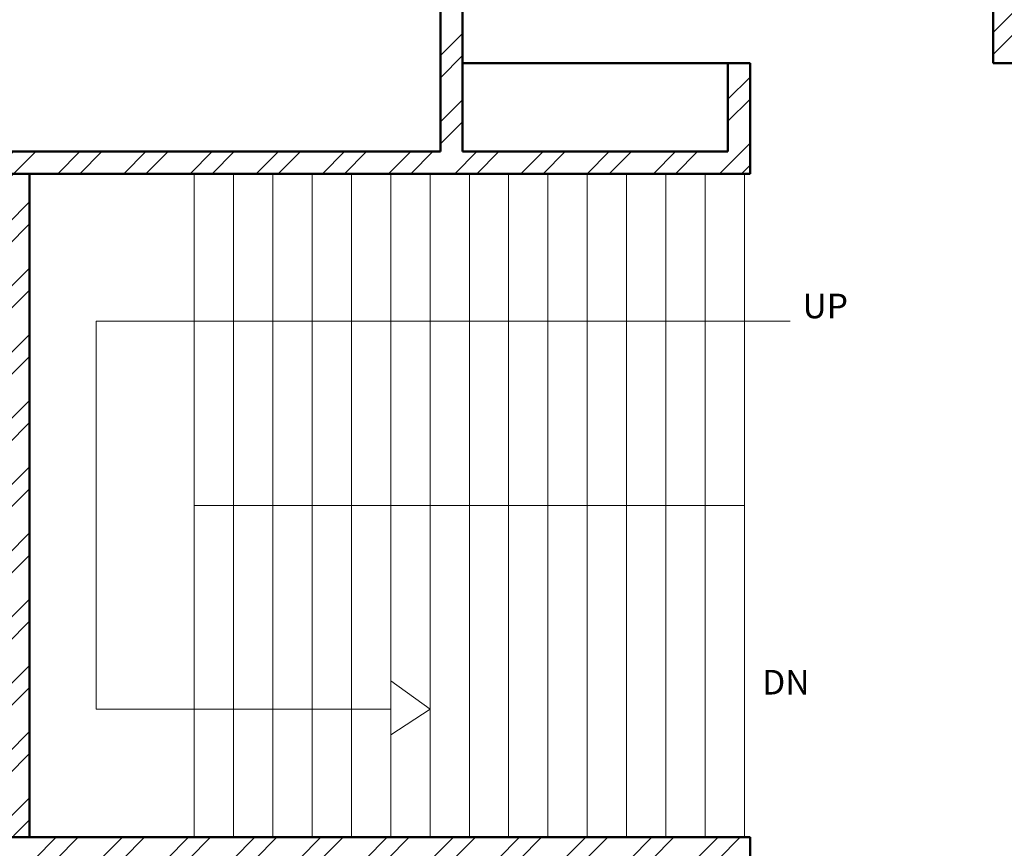
# Model space of a CAD drawing. Units: inches. Extents: x 963 to 2075, y 289 to 2657.
# Tile 29 of 98: x 1310 to 1511, y 1949 to 2117. Entities that reach past the tile are written whole.
import ezdxf

# ---------------------------------------------------------------- set-up
doc = ezdxf.new("R2010")
doc.units = ezdxf.units.IN
for name, color, linetype, lineweight in [('A-AREA-IDEN', 7, 'Continuous', 18), ('A-FLOR-STRS', 2, 'Continuous', 18), ('A-WALL', 7, 'Continuous', 50), ('A-WALL-PATT', 8, 'Continuous', 13)]:
    doc.layers.add(name, color=color, linetype=linetype, lineweight=lineweight)
doc.styles.get("Standard").update_dxf_attribs({"font": 'arial.ttf'})

msp = doc.modelspace()

# ---------------------------------------------------------------- hatches: boundary and pattern name
at = {"layer": 'A-WALL-PATT'}
h = msp.add_hatch(dxfattribs=at)
h.set_pattern_fill('ANSI32', color=256)
h.paths.add_polyline_path([(1296.92, 2558.32), (1203.92, 2558.32), (1203.92, 2493.82), (1191.53, 2493.82), (1191.53, 2489.32), (1211.06, 2489.32), (1211.06, 2492.02), (1211.06, 2493.82), (1208.42, 2493.82), (1208.42, 2553.82), (1292.42, 2553.82), (1292.42, 2538.86), (1296.92, 2538.86)])
h.paths.add_polyline_path([(1442.42, 2558.32), (1349.42, 2558.32), (1349.42, 2538.94), (1353.92, 2538.94), (1353.92, 2553.82), (1437.92, 2553.82), (1437.92, 2493.82), (1434.54, 2493.82), (1434.54, 2489.32), (1448.31, 2489.32), (1448.31, 2491.57), (1448.31, 2493.82), (1442.42, 2493.82)])
h.paths.add_polyline_path([(1415.55, 2491.57), (1415.55, 2493.82), (1340.94, 2493.82), (1340.94, 2489.32), (1371.92, 2489.32), (1371.92, 2378.32), (1367.6, 2378.32), (1367.6, 2373.82), (1371.92, 2373.82), (1371.92, 2355.19), (1376.42, 2355.19), (1376.42, 2489.32), (1415.55, 2489.32)])
h.paths.add_polyline_path([(1304.94, 2491.57), (1304.94, 2493.82), (1296.92, 2493.82), (1296.92, 2514.86), (1292.42, 2514.86), (1292.42, 2493.82), (1232.81, 2493.82), (1232.81, 2489.32), (1256.42, 2489.32), (1256.42, 2327.32), (1253.71, 2327.32), (1253.71, 2322.82), (1328.42, 2322.82), (1328.42, 2331.15), (1323.92, 2331.15), (1323.92, 2327.32), (1260.92, 2327.32), (1260.92, 2373.82), (1323.92, 2373.82), (1323.92, 2357.81), (1328.42, 2357.81), (1328.42, 2373.82), (1346.01, 2373.82), (1346.01, 2376.07), (1346.01, 2378.32), (1260.92, 2378.32), (1260.92, 2489.32), (1304.94, 2489.32)])
h.paths.add_polyline_path([(1226.65, 2327.32), (1124.42, 2327.32), (1124.42, 2347.45), (1119.92, 2347.45), (1119.92, 2322.82), (1163.42, 2322.82), (1163.42, 2305.43), (1165.67, 2305.43), (1167.92, 2305.43), (1167.92, 2322.82), (1226.65, 2322.82), (1226.65, 2325.07)])
h.paths.add_polyline_path([(1095.92, 2489.32), (1124.42, 2489.32), (1131.53, 2489.32), (1131.53, 2491.57), (1131.53, 2493.82), (1119.92, 2493.82), (1091.42, 2493.82), (1091.42, 2417.32), (1095.92, 2417.32), (1119.92, 2417.32), (1119.92, 2407.45), (1124.42, 2407.45), (1124.42, 2421.82), (1095.92, 2421.82)])
h.paths.add_polyline_path([(1512.92, 2558.32), (1508.42, 2558.32), (1508.42, 2493.82), (1503.4, 2493.82), (1503.4, 2489.32), (1508.42, 2489.32), (1508.42, 2327.32), (1376.42, 2327.32), (1376.42, 2330.27), (1371.92, 2330.27), (1371.92, 2298.74), (1376.42, 2298.74), (1376.42, 2322.82), (1508.42, 2322.82), (1508.42, 2165.32), (1504.26, 2165.32), (1504.26, 2160.82), (1508.42, 2160.82), (1508.42, 2108.32), (1512.92, 2108.32), (1512.92, 2160.82), (1516.18, 2160.82), (1516.18, 2163.07), (1516.18, 2165.32), (1512.92, 2165.32), (1512.92, 2322.82), (1644.92, 2322.82), (1644.92, 2298.74), (1649.42, 2298.74), (1649.42, 2322.82), (1649.42, 2330.94), (1647.17, 2330.94), (1644.92, 2330.94), (1644.92, 2327.32), (1512.92, 2327.32), (1512.92, 2489.32), (1516.76, 2489.32), (1516.76, 2491.57), (1516.76, 2493.82), (1512.92, 2493.82)])
h.paths.add_polyline_path([(1671.92, 2558.32), (1578.92, 2558.32), (1578.92, 2493.82), (1573.53, 2493.82), (1573.53, 2489.32), (1586.54, 2489.32), (1586.54, 2491.57), (1586.54, 2493.82), (1583.42, 2493.82), (1583.42, 2553.82), (1667.42, 2553.82), (1667.42, 2541.11), (1671.92, 2541.11)])
h.paths.add_polyline_path([(1681.26, 2493.82), (1671.92, 2493.82), (1671.92, 2517.11), (1667.42, 2517.11), (1667.42, 2493.82), (1610.22, 2493.82), (1610.22, 2489.32), (1644.92, 2489.32), (1644.92, 2357.87), (1649.42, 2357.87), (1649.42, 2373.82), (1652.2, 2373.82), (1652.2, 2375.83), (1652.2, 2378.32), (1649.42, 2378.32), (1649.42, 2489.32), (1681.26, 2489.32), (1681.26, 2491.57)])
h.paths.add_polyline_path([(1821.92, 2558.32), (1728.92, 2558.32), (1728.92, 2541), (1733.42, 2541), (1733.42, 2553.82), (1817.42, 2553.82), (1817.42, 2493.82), (1813.51, 2493.82), (1813.51, 2489.32), (1830.08, 2489.32), (1830.08, 2491.57), (1830.08, 2493.82), (1821.92, 2493.82)])
h.paths.add_polyline_path([(1794.24, 2493.82), (1717.26, 2493.82), (1717.26, 2489.32), (1760.42, 2489.32), (1760.42, 2378.32), (1674.4, 2378.32), (1674.4, 2373.82), (1692.92, 2373.82), (1692.92, 2356.95), (1697.42, 2356.95), (1697.42, 2373.82), (1760.42, 2373.82), (1760.42, 2327.32), (1697.42, 2327.32), (1697.42, 2333.34), (1692.92, 2333.34), (1692.92, 2322.82), (1768.04, 2322.82), (1768.04, 2325.07), (1768.04, 2327.32), (1764.92, 2327.32), (1764.92, 2489.32), (1794.24, 2489.32)])
h.paths.add_polyline_path([(1733.42, 2517), (1728.92, 2517), (1728.92, 2493.82), (1733.42, 2493.82)], flags=17)
h.paths.add_polyline_path([(1929.92, 2493.82), (1890.08, 2493.82), (1890.08, 2489.32), (1896.92, 2489.32), (1925.42, 2489.32), (1925.42, 2421.82), (1896.92, 2421.82), (1896.92, 2408.32), (1901.42, 2408.32), (1901.42, 2417.32), (1925.42, 2417.32), (1929.92, 2417.32)])
h.paths.add_polyline_path([(1901.42, 2348.32), (1896.92, 2348.32), (1896.92, 2327.32), (1800.42, 2327.32), (1800.42, 2322.82), (1853.42, 2322.82), (1853.42, 2309.45), (1857.92, 2309.45), (1857.92, 2322.82), (1901.42, 2322.82)])
h.paths.add_polyline_path([(1857.92, 2249.45), (1853.42, 2249.45), (1853.42, 2214.82), (1686.31, 2214.82), (1686.31, 2210.32), (1853.42, 2210.32), (1853.42, 2202.13), (1857.92, 2202.13), (1857.92, 2210.32)])
h.paths.add_polyline_path([(1857.92, 2142.13), (1853.42, 2142.13), (1853.42, 2115.42), (1841.42, 2115.42), (1841.42, 2088.53), (1841.42, 2046.95), (1845.92, 2046.95), (1845.92, 2110.92), (1905.92, 2110.92), (1905.92, 2092.52), (1910.42, 2092.52), (1910.42, 2115.42), (1857.92, 2115.42)])
h.paths.add_polyline_path([(1532.44, 1482.34), (1573.46, 1482.34), (1573.46, 1501), (1532.44, 1501)], flags=9)
h.paths.add_polyline_path([(1438.66, 1486.3), (1479.68, 1486.3), (1479.68, 1504.96), (1438.66, 1504.96)], flags=9)
h.paths.add_polyline_path([(1411.22, 1365.31), (1659.14, 1365.31), (1659.14, 1402.4), (1411.22, 1402.4)], flags=9)
h.paths.add_polyline_path([(1185.67, 2296.3), (1248.16, 2296.3), (1248.16, 2314.95), (1185.67, 2314.95)], flags=9)
h.paths.add_polyline_path([(1177.31, 2187.35), (1216.15, 2187.35), (1216.15, 2206.01), (1177.31, 2206.01)], flags=9)
h.paths.add_polyline_path([(1295.1, 1602.08), (1328.26, 1602.08), (1328.26, 1620.74), (1295.1, 1620.74)], flags=9)
h.paths.add_polyline_path([(1525.13, 2005.99), (1558.39, 2005.99), (1558.39, 2024.65), (1525.13, 2024.65)], flags=9)
h.paths.add_polyline_path([(1459.61, 1977.13), (1472.19, 1977.13), (1472.19, 1987.43), (1459.61, 1987.43)], flags=9)
h.paths.add_polyline_path([(1467.81, 2053.68), (1480.02, 2053.68), (1480.02, 2063.98), (1467.81, 2063.98)], flags=9)
h.paths.add_polyline_path([(1555.18, 2119.02), (1584.56, 2119.02), (1584.56, 2137.68), (1555.18, 2137.68)], flags=25)
h.paths.add_polyline_path([(1405.39, 2115.29), (1444.48, 2115.29), (1444.48, 2133.95), (1405.39, 2133.95)], flags=25)
h.paths.add_polyline_path([(1698.48, 2004.26), (1727.69, 2004.26), (1727.69, 2022.92), (1698.48, 2022.92)], flags=9)
h.paths.add_polyline_path([(1612.16, 1972.86), (1629.02, 1972.86), (1629.02, 1983.16), (1612.16, 1983.16)], flags=9)
h.paths.add_polyline_path([(1608.29, 2060.04), (1625.15, 2060.04), (1625.15, 2070.34), (1608.29, 2070.34)], flags=9)
h.paths.add_polyline_path([(1527.95, 1684.4), (1566.79, 1684.4), (1566.79, 1703.06), (1527.95, 1703.06)], flags=9)
h.paths.add_polyline_path([(1422.79, 1683.59), (1461.63, 1683.59), (1461.63, 1702.25), (1422.79, 1702.25)], flags=9)
h.paths.add_polyline_path([(1531.26, 1732.46), (1574.01, 1732.46), (1574.01, 1751.12), (1531.26, 1751.12)], flags=9)
h.paths.add_polyline_path([(1402.87, 1732.85), (1439.8, 1732.85), (1439.8, 1751.5), (1402.87, 1751.5)], flags=9)
h.paths.add_polyline_path([(1243.12, 1923.13), (1281.96, 1923.13), (1281.96, 1941.79), (1243.12, 1941.79)], flags=9)
h.paths.add_polyline_path([(1181.75, 1792.27), (1244.24, 1792.27), (1244.24, 1810.93), (1181.75, 1810.93)], flags=9)
h.paths.add_polyline_path([(1265.82, 1670.3), (1316.07, 1670.3), (1316.07, 1688.96), (1265.82, 1688.96)], flags=9)
h.paths.add_polyline_path([(1140.26, 1676.05), (1179.1, 1676.05), (1179.1, 1694.71), (1140.26, 1694.71)], flags=9)
h.paths.add_polyline_path([(1107.49, 1490.89), (1143.37, 1490.89), (1143.37, 1509.55), (1107.49, 1509.55)], flags=9)
h.paths.add_polyline_path([(1217.58, 1483.9), (1246.74, 1483.9), (1246.74, 1502.56), (1217.58, 1502.56)], flags=9)
h.paths.add_polyline_path([(1389.21, 1486.92), (1418.37, 1486.92), (1418.37, 1505.58), (1389.21, 1505.58)], flags=9)
h.paths.add_polyline_path([(1672.21, 1602.08), (1705.37, 1602.08), (1705.37, 1620.74), (1672.21, 1620.74)], flags=9)
h.paths.add_polyline_path([(1752.08, 1522.64), (1781.24, 1522.64), (1781.24, 1541.3), (1752.08, 1541.3)], flags=9)
h.paths.add_polyline_path([(1848.27, 1491.26), (1884.16, 1491.26), (1884.16, 1509.92), (1848.27, 1509.92)], flags=9)
h.paths.add_polyline_path([(1822.47, 1685.62), (1861.31, 1685.62), (1861.31, 1704.28), (1822.47, 1704.28)], flags=9)
h.paths.add_polyline_path([(1713.19, 1672.23), (1763.44, 1672.23), (1763.44, 1690.89), (1713.19, 1690.89)], flags=9)
h.paths.add_polyline_path([(1736.62, 1790.58), (1799.11, 1790.58), (1799.11, 1809.24), (1736.62, 1809.24)], flags=9)
h.paths.add_polyline_path([(1691.49, 1916.36), (1730.33, 1916.36), (1730.33, 1935.01), (1691.49, 1935.01)], flags=9)
h.paths.add_polyline_path([(1764.87, 1973.92), (1794.31, 1973.92), (1794.31, 1992.58), (1764.87, 1992.58)], flags=9)
h.paths.add_polyline_path([(1767.85, 2034.02), (1797.29, 2034.02), (1797.29, 2052.67), (1767.85, 2052.67)], flags=9)
h.paths.add_polyline_path([(1851.59, 2060.33), (1880.75, 2060.33), (1880.75, 2078.99), (1851.59, 2078.99)], flags=25)
h.paths.add_polyline_path([(1688.49, 2086.87), (1727.33, 2086.87), (1727.33, 2105.53), (1688.49, 2105.53)], flags=9)
h.paths.add_polyline_path([(1537.74, 2293.58), (1580.49, 2293.58), (1580.49, 2312.24), (1537.74, 2312.24)], flags=25)
h.paths.add_polyline_path([(1425.59, 2296.11), (1468.34, 2296.11), (1468.34, 2314.77), (1425.59, 2314.77)], flags=25)
h.paths.add_polyline_path([(1278.52, 2004.18), (1307.72, 2004.18), (1307.72, 2022.84), (1278.52, 2022.84)], flags=9)
h.paths.add_polyline_path([(1193.28, 1973.63), (1222.72, 1973.63), (1222.72, 1992.29), (1193.28, 1992.29)], flags=9)
h.paths.add_polyline_path([(1192.41, 2040.58), (1221.84, 2040.58), (1221.84, 2059.23), (1192.41, 2059.23)], flags=9)
h.paths.add_polyline_path([(1130.6, 1951.39), (1159.76, 1951.39), (1159.76, 1970.05), (1130.6, 1970.05)], flags=9)
h.paths.add_polyline_path([(1132.83, 2052.49), (1161.98, 2052.49), (1161.98, 2071.15), (1132.83, 2071.15)], flags=9)
h.paths.add_polyline_path([(1265.13, 2334.62), (1315.38, 2334.62), (1315.38, 2353.28), (1265.13, 2353.28)], flags=25)
h.paths.add_polyline_path([(1136.74, 2330.79), (1175.58, 2330.79), (1175.58, 2349.44), (1136.74, 2349.44)], flags=9)
h.paths.add_polyline_path([(1287.42, 2417.2), (1320.58, 2417.2), (1320.58, 2435.86), (1287.42, 2435.86)], flags=25)
h.paths.add_polyline_path([(1430.99, 2329.16), (1469.83, 2329.16), (1469.83, 2347.82), (1430.99, 2347.82)], flags=25)
h.paths.add_polyline_path([(1525.42, 2329.21), (1564.26, 2329.21), (1564.26, 2347.87), (1525.42, 2347.87)], flags=25)
h.paths.add_polyline_path([(1684.52, 2382.8), (1717.68, 2382.8), (1717.68, 2401.46), (1684.52, 2401.46)], flags=25)
h.paths.add_polyline_path([(1704.81, 2340.29), (1755.05, 2340.29), (1755.05, 2358.95), (1704.81, 2358.95)], flags=25)
h.paths.add_polyline_path([(1694.11, 2287.76), (1756.6, 2287.76), (1756.6, 2306.41), (1694.11, 2306.41)], flags=9)
h.paths.add_polyline_path([(1815.78, 2329.86), (1854.62, 2329.86), (1854.62, 2348.52), (1815.78, 2348.52)], flags=9)
h.paths.add_polyline_path([(1842.87, 2514.26), (1878.76, 2514.26), (1878.76, 2532.91), (1842.87, 2532.91)], flags=9)
h.paths.add_polyline_path([(1769.51, 2531.45), (1798.67, 2531.45), (1798.67, 2550.1), (1769.51, 2550.1)], flags=25)
h.paths.add_polyline_path([(1594.77, 2518.47), (1623.93, 2518.47), (1623.93, 2537.13), (1594.77, 2537.13)], flags=25)
h.paths.add_polyline_path([(1520.72, 2516.18), (1556.61, 2516.18), (1556.61, 2534.84), (1520.72, 2534.84)], flags=25)
h.paths.add_polyline_path([(1464.46, 2516.69), (1500.34, 2516.69), (1500.34, 2535.35), (1464.46, 2535.35)], flags=25)
h.paths.add_polyline_path([(1365.7, 2528.97), (1394.85, 2528.97), (1394.85, 2547.63), (1365.7, 2547.63)], flags=25)
h.paths.add_polyline_path([(1222.84, 2516.23), (1252, 2516.23), (1252, 2534.89), (1222.84, 2534.89)], flags=25)
h.paths.add_polyline_path([(1104.55, 2509.6), (1140.43, 2509.6), (1140.43, 2528.26), (1104.55, 2528.26)], flags=9)
h = msp.add_hatch(dxfattribs=at)
h.set_pattern_fill('ANSI32', color=256)
h.paths.add_polyline_path([(1335.97, 2212.57), (1335.97, 2214.82), (1167.92, 2214.82), (1167.92, 2245.43), (1163.42, 2245.43), (1163.42, 2210.32), (1163.42, 2194.81), (1167.92, 2194.81), (1167.92, 2210.32), (1335.97, 2210.32)])
h.paths.add_polyline_path([(1532.44, 1482.34), (1573.46, 1482.34), (1573.46, 1501), (1532.44, 1501)], flags=9)
h.paths.add_polyline_path([(1438.66, 1486.3), (1479.68, 1486.3), (1479.68, 1504.96), (1438.66, 1504.96)], flags=9)
h.paths.add_polyline_path([(1411.22, 1365.31), (1659.14, 1365.31), (1659.14, 1402.4), (1411.22, 1402.4)], flags=9)
h.paths.add_polyline_path([(1185.67, 2296.3), (1248.16, 2296.3), (1248.16, 2314.95), (1185.67, 2314.95)], flags=9)
h.paths.add_polyline_path([(1177.31, 2187.35), (1216.15, 2187.35), (1216.15, 2206.01), (1177.31, 2206.01)], flags=9)
h.paths.add_polyline_path([(1295.1, 1602.08), (1328.26, 1602.08), (1328.26, 1620.74), (1295.1, 1620.74)], flags=9)
h.paths.add_polyline_path([(1525.13, 2005.99), (1558.39, 2005.99), (1558.39, 2024.65), (1525.13, 2024.65)], flags=9)
h.paths.add_polyline_path([(1459.61, 1977.13), (1472.19, 1977.13), (1472.19, 1987.43), (1459.61, 1987.43)], flags=9)
h.paths.add_polyline_path([(1467.81, 2053.68), (1480.02, 2053.68), (1480.02, 2063.98), (1467.81, 2063.98)], flags=9)
h.paths.add_polyline_path([(1555.18, 2119.02), (1584.56, 2119.02), (1584.56, 2137.68), (1555.18, 2137.68)], flags=9)
h.paths.add_polyline_path([(1405.39, 2115.29), (1444.48, 2115.29), (1444.48, 2133.95), (1405.39, 2133.95)], flags=9)
h.paths.add_polyline_path([(1698.48, 2004.26), (1727.69, 2004.26), (1727.69, 2022.92), (1698.48, 2022.92)], flags=9)
h.paths.add_polyline_path([(1612.16, 1972.86), (1629.02, 1972.86), (1629.02, 1983.16), (1612.16, 1983.16)], flags=9)
h.paths.add_polyline_path([(1608.29, 2060.04), (1625.15, 2060.04), (1625.15, 2070.34), (1608.29, 2070.34)], flags=9)
h.paths.add_polyline_path([(1527.95, 1684.4), (1566.79, 1684.4), (1566.79, 1703.06), (1527.95, 1703.06)], flags=9)
h.paths.add_polyline_path([(1422.79, 1683.59), (1461.63, 1683.59), (1461.63, 1702.25), (1422.79, 1702.25)], flags=9)
h.paths.add_polyline_path([(1531.26, 1732.46), (1574.01, 1732.46), (1574.01, 1751.12), (1531.26, 1751.12)], flags=9)
h.paths.add_polyline_path([(1402.87, 1732.85), (1439.8, 1732.85), (1439.8, 1751.5), (1402.87, 1751.5)], flags=9)
h.paths.add_polyline_path([(1243.12, 1923.13), (1281.96, 1923.13), (1281.96, 1941.79), (1243.12, 1941.79)], flags=9)
h.paths.add_polyline_path([(1181.75, 1792.27), (1244.24, 1792.27), (1244.24, 1810.93), (1181.75, 1810.93)], flags=9)
h.paths.add_polyline_path([(1265.82, 1670.3), (1316.07, 1670.3), (1316.07, 1688.96), (1265.82, 1688.96)], flags=9)
h.paths.add_polyline_path([(1140.26, 1676.05), (1179.1, 1676.05), (1179.1, 1694.71), (1140.26, 1694.71)], flags=9)
h.paths.add_polyline_path([(1107.49, 1490.89), (1143.37, 1490.89), (1143.37, 1509.55), (1107.49, 1509.55)], flags=9)
h.paths.add_polyline_path([(1217.58, 1483.9), (1246.74, 1483.9), (1246.74, 1502.56), (1217.58, 1502.56)], flags=9)
h.paths.add_polyline_path([(1389.21, 1486.92), (1418.37, 1486.92), (1418.37, 1505.58), (1389.21, 1505.58)], flags=9)
h.paths.add_polyline_path([(1672.21, 1602.08), (1705.37, 1602.08), (1705.37, 1620.74), (1672.21, 1620.74)], flags=9)
h.paths.add_polyline_path([(1752.08, 1522.64), (1781.24, 1522.64), (1781.24, 1541.3), (1752.08, 1541.3)], flags=9)
h.paths.add_polyline_path([(1848.27, 1491.26), (1884.16, 1491.26), (1884.16, 1509.92), (1848.27, 1509.92)], flags=9)
h.paths.add_polyline_path([(1822.47, 1685.62), (1861.31, 1685.62), (1861.31, 1704.28), (1822.47, 1704.28)], flags=9)
h.paths.add_polyline_path([(1713.19, 1672.23), (1763.44, 1672.23), (1763.44, 1690.89), (1713.19, 1690.89)], flags=9)
h.paths.add_polyline_path([(1736.62, 1790.58), (1799.11, 1790.58), (1799.11, 1809.24), (1736.62, 1809.24)], flags=9)
h.paths.add_polyline_path([(1691.49, 1916.36), (1730.33, 1916.36), (1730.33, 1935.01), (1691.49, 1935.01)], flags=9)
h.paths.add_polyline_path([(1764.87, 1973.92), (1794.31, 1973.92), (1794.31, 1992.58), (1764.87, 1992.58)], flags=9)
h.paths.add_polyline_path([(1767.85, 2034.02), (1797.29, 2034.02), (1797.29, 2052.67), (1767.85, 2052.67)], flags=9)
h.paths.add_polyline_path([(1851.59, 2060.33), (1880.75, 2060.33), (1880.75, 2078.99), (1851.59, 2078.99)], flags=9)
h.paths.add_polyline_path([(1688.49, 2086.87), (1727.33, 2086.87), (1727.33, 2105.53), (1688.49, 2105.53)], flags=9)
h.paths.add_polyline_path([(1537.74, 2293.58), (1580.49, 2293.58), (1580.49, 2312.24), (1537.74, 2312.24)], flags=9)
h.paths.add_polyline_path([(1425.59, 2296.11), (1468.34, 2296.11), (1468.34, 2314.77), (1425.59, 2314.77)], flags=9)
h.paths.add_polyline_path([(1278.52, 2004.18), (1307.72, 2004.18), (1307.72, 2022.84), (1278.52, 2022.84)], flags=9)
h.paths.add_polyline_path([(1193.28, 1973.63), (1222.72, 1973.63), (1222.72, 1992.29), (1193.28, 1992.29)], flags=9)
h.paths.add_polyline_path([(1192.41, 2040.58), (1221.84, 2040.58), (1221.84, 2059.23), (1192.41, 2059.23)], flags=9)
h.paths.add_polyline_path([(1130.6, 1951.39), (1159.76, 1951.39), (1159.76, 1970.05), (1130.6, 1970.05)], flags=9)
h.paths.add_polyline_path([(1132.83, 2052.49), (1161.98, 2052.49), (1161.98, 2071.15), (1132.83, 2071.15)], flags=9)
h.paths.add_polyline_path([(1265.13, 2334.62), (1315.38, 2334.62), (1315.38, 2353.28), (1265.13, 2353.28)], flags=9)
h.paths.add_polyline_path([(1136.74, 2330.79), (1175.58, 2330.79), (1175.58, 2349.44), (1136.74, 2349.44)], flags=9)
h.paths.add_polyline_path([(1287.42, 2417.2), (1320.58, 2417.2), (1320.58, 2435.86), (1287.42, 2435.86)], flags=9)
h.paths.add_polyline_path([(1430.99, 2329.16), (1469.83, 2329.16), (1469.83, 2347.82), (1430.99, 2347.82)], flags=9)
h.paths.add_polyline_path([(1525.42, 2329.21), (1564.26, 2329.21), (1564.26, 2347.87), (1525.42, 2347.87)], flags=9)
h.paths.add_polyline_path([(1684.52, 2382.8), (1717.68, 2382.8), (1717.68, 2401.46), (1684.52, 2401.46)], flags=9)
h.paths.add_polyline_path([(1704.81, 2340.29), (1755.05, 2340.29), (1755.05, 2358.95), (1704.81, 2358.95)], flags=9)
h.paths.add_polyline_path([(1694.11, 2287.76), (1756.6, 2287.76), (1756.6, 2306.41), (1694.11, 2306.41)], flags=9)
h.paths.add_polyline_path([(1815.78, 2329.86), (1854.62, 2329.86), (1854.62, 2348.52), (1815.78, 2348.52)], flags=9)
h.paths.add_polyline_path([(1842.87, 2514.26), (1878.76, 2514.26), (1878.76, 2532.91), (1842.87, 2532.91)], flags=9)
h.paths.add_polyline_path([(1769.51, 2531.45), (1798.67, 2531.45), (1798.67, 2550.1), (1769.51, 2550.1)], flags=9)
h.paths.add_polyline_path([(1594.77, 2518.47), (1623.93, 2518.47), (1623.93, 2537.13), (1594.77, 2537.13)], flags=9)
h.paths.add_polyline_path([(1520.72, 2516.18), (1556.61, 2516.18), (1556.61, 2534.84), (1520.72, 2534.84)], flags=9)
h.paths.add_polyline_path([(1464.46, 2516.69), (1500.34, 2516.69), (1500.34, 2535.35), (1464.46, 2535.35)], flags=9)
h.paths.add_polyline_path([(1365.7, 2528.97), (1394.85, 2528.97), (1394.85, 2547.63), (1365.7, 2547.63)], flags=9)
h.paths.add_polyline_path([(1222.84, 2516.23), (1252, 2516.23), (1252, 2534.89), (1222.84, 2534.89)], flags=9)
h.paths.add_polyline_path([(1104.55, 2509.6), (1140.43, 2509.6), (1140.43, 2528.26), (1104.55, 2528.26)], flags=9)
h = msp.add_hatch(dxfattribs=at)
h.set_pattern_fill('ANSI32', color=256)
h.paths.add_polyline_path([(1473.61, 2163.07), (1473.61, 2165.32), (1376.42, 2165.32), (1376.42, 2227.98), (1371.92, 2227.98), (1371.92, 2214.82), (1368.41, 2214.82), (1368.41, 2210.32), (1371.92, 2210.32), (1371.92, 2160.82), (1395.92, 2160.82), (1395.92, 2090.32), (1217.34, 2090.32), (1217.34, 2085.82), (1395.92, 2085.82), (1458.92, 2085.82), (1458.92, 2108.32), (1454.42, 2108.32), (1454.42, 2090.32), (1400.42, 2090.32), (1400.42, 2160.82), (1473.61, 2160.82)])
h.paths.add_polyline_path([(1649.42, 2210.32), (1653.23, 2210.32), (1653.23, 2214.82), (1649.42, 2214.82), (1649.42, 2227.98), (1644.92, 2227.98), (1644.92, 2165.32), (1550.1, 2165.32), (1550.1, 2160.82), (1620.92, 2160.82), (1620.92, 2112.82), (1555.45, 2112.82), (1555.45, 2108.32), (1584.33, 2108.32), (1584.33, 2084.92), (1588.83, 2084.92), (1588.83, 2108.32), (1625.42, 2108.32), (1667.95, 2108.32), (1667.95, 2022.67), (1588.83, 2022.67), (1588.83, 2047.41), (1584.33, 2047.41), (1584.33, 1996), (1588.83, 1996), (1588.83, 2018.32), (1667.95, 2018.17), (1667.95, 1928.32), (1625.42, 1928.32), (1625.42, 1923.82), (1672.45, 1923.82), (1672.45, 1928.32), (1672.45, 1946.66), (1785.45, 1946.66), (1785.45, 1951.16), (1743.03, 1951.16), (1743.03, 2017.92), (1841.42, 2017.92), (1841.42, 2014.77), (1845.92, 2014.77), (1845.92, 2017.92), (1905.92, 2017.92), (1905.92, 1987.51), (1910.42, 1987.51), (1910.42, 2022.42), (1910.42, 2068.52), (1905.92, 2068.52), (1905.92, 2022.42), (1845.92, 2022.42), (1845.92, 2025.85), (1843.67, 2025.85), (1841.42, 2025.85), (1841.42, 2022.42), (1743.03, 2022.42), (1743.03, 2084.03), (1768.45, 2084.03), (1785.45, 2084.03), (1785.45, 2088.53), (1672.45, 2088.53), (1672.45, 2112.82), (1667.95, 2112.82), (1625.42, 2112.82), (1625.42, 2160.82), (1649.42, 2160.82)])
h.paths.add_polyline_path([(1672.45, 2084.03), (1738.53, 2084.03), (1738.53, 1951.16), (1672.45, 1951.16)], flags=16)
h.paths.add_polyline_path([(1672.45, 2084.03), (1738.53, 2084.03), (1705.49, 2017.6)], flags=0)
h.paths.add_polyline_path([(1262.77, 2085.82), (1258.27, 2085.82), (1258.27, 2023.28), (1184.42, 2023.28), (1184.42, 2018.78), (1258.27, 2018.78), (1258.27, 1950.82), (1262.77, 1950.82)])
h.paths.add_polyline_path([(1312.27, 2085.82), (1307.77, 2085.82), (1307.77, 1950.82), (1312.27, 1950.82)])
h.paths.add_polyline_path([(1458.92, 1950.82), (1395.92, 1950.82), (1216.57, 1950.82), (1216.57, 1946.32), (1346.42, 1946.32), (1395.92, 1946.32), (1395.92, 1875.82), (1371.92, 1875.82), (1371.92, 1826.32), (1368.93, 1826.32), (1368.93, 1821.82), (1371.92, 1821.82), (1371.92, 1813.62), (1376.42, 1813.62), (1376.42, 1871.32), (1474.5, 1871.32), (1474.5, 1873.57), (1474.5, 1875.82), (1400.42, 1875.82), (1400.42, 1946.32), (1454.42, 1946.32), (1454.42, 1928.32), (1458.92, 1928.32)])
h.paths.add_polyline_path([(1184.42, 2120.78), (1167.92, 2120.78), (1167.92, 2134.81), (1165.67, 2134.81), (1163.42, 2134.81), (1163.42, 2120.78), (1119.92, 2120.78), (1119.92, 2098.1), (1124.42, 2098.1), (1124.42, 2116.28), (1167.92, 2116.28), (1179.92, 2116.28), (1179.92, 2045.92), (1184.42, 2045.92), (1184.42, 2090.32), (1184.42, 2116.28)])
h.paths.add_polyline_path([(1124.42, 2018.78), (1179.92, 2018.78), (1179.92, 2016.29), (1184.42, 2016.29), (1184.42, 2023.28), (1184.42, 2026.59), (1182.17, 2026.59), (1179.92, 2026.59), (1179.92, 2023.28), (1124.42, 2023.28), (1124.42, 2074.1), (1119.92, 2074.1), (1119.92, 2018.78), (1119.92, 1979.63), (1124.42, 1979.63)])
h.paths.add_polyline_path([(1184.42, 1925.78), (1184.42, 1946.32), (1184.42, 1996.07), (1182.17, 1996.07), (1179.92, 1996.07), (1179.92, 1925.78), (1124.42, 1925.78), (1124.42, 1955.63), (1119.92, 1955.5), (1119.92, 1921.28), (1158.92, 1921.28), (1158.92, 1909.98), (1163.42, 1909.98), (1163.42, 1921.28), (1184.42, 1921.28)])
h.paths.add_polyline_path([(1341.45, 1826.32), (1163.42, 1826.32), (1163.42, 1849.98), (1158.92, 1849.98), (1158.92, 1821.82), (1158.92, 1804.03), (1163.42, 1804.03), (1163.42, 1821.82), (1341.45, 1821.82)])
h.paths.add_polyline_path([(1222.98, 1713.82), (1163.42, 1713.82), (1163.42, 1744.03), (1161.17, 1744.03), (1158.92, 1744.03), (1158.92, 1713.82), (1119.92, 1713.82), (1119.92, 1694.65), (1124.42, 1694.65), (1124.42, 1709.32), (1158.92, 1709.32), (1222.98, 1709.32)])
h.paths.add_polyline_path([(1328.42, 1713.82), (1252.04, 1713.82), (1252.04, 1711.57), (1252.04, 1709.32), (1256.42, 1709.32), (1256.42, 1547.32), (1232.94, 1547.32), (1232.94, 1545.07), (1232.94, 1542.82), (1292.42, 1542.82), (1292.42, 1527.63), (1296.92, 1527.63), (1296.92, 1542.82), (1299.46, 1542.82), (1299.46, 1547.32), (1260.92, 1547.32), (1260.92, 1658.32), (1343.66, 1658.32), (1343.66, 1660.57), (1343.66, 1662.82), (1328.42, 1662.82), (1328.42, 1676.59), (1327.4, 1676.59), (1323.92, 1676.59), (1323.92, 1662.82), (1260.92, 1662.82), (1260.92, 1709.32), (1323.92, 1709.32), (1323.92, 1699.85), (1328.42, 1699.85)])
h.paths.add_polyline_path([(1649.42, 1875.82), (1625.42, 1875.82), (1625.42, 1928.32), (1620.92, 1928.32), (1588.83, 1928.32), (1588.83, 1950.59), (1584.33, 1950.59), (1584.33, 1928.32), (1555.45, 1928.32), (1555.45, 1923.82), (1620.92, 1923.82), (1620.92, 1875.82), (1548.95, 1875.82), (1548.95, 1873.57), (1548.95, 1871.32), (1644.92, 1871.32), (1644.92, 1813.62), (1649.42, 1813.62), (1649.42, 1821.82), (1652.04, 1821.82), (1652.04, 1824.07), (1652.04, 1826.32), (1649.42, 1826.32)])
h.paths.add_polyline_path([(1512.92, 1871.32), (1516.48, 1871.32), (1516.48, 1875.82), (1512.92, 1875.82), (1512.92, 1923.82), (1512.92, 1928.32), (1512.92, 1930.83), (1508.42, 1930.83), (1508.42, 1875.82), (1504.41, 1875.82), (1504.41, 1871.32), (1508.42, 1871.32), (1508.42, 1713.82), (1376.42, 1713.82), (1376.42, 1743.32), (1371.92, 1743.32), (1371.92, 1709.32), (1371.92, 1706.01), (1376.42, 1706.01), (1376.42, 1709.32), (1508.42, 1709.32), (1508.42, 1547.32), (1501.87, 1547.32), (1501.87, 1542.82), (1508.42, 1542.82), (1508.42, 1482.82), (1508.42, 1436.32), (1512.92, 1436.32), (1512.92, 1542.82), (1519.32, 1542.82), (1519.32, 1545.07), (1519.32, 1547.32), (1512.92, 1547.32), (1512.92, 1709.32), (1644.92, 1709.32), (1644.92, 1707.55), (1649.42, 1707.55), (1649.42, 1709.32), (1649.42, 1743.32), (1644.92, 1743.32), (1644.92, 1713.82), (1512.92, 1713.82)])
h.paths.add_polyline_path([(1129.88, 1545.07), (1129.88, 1547.32), (1124.42, 1547.32), (1095.92, 1547.32), (1095.92, 1614.82), (1124.42, 1614.82), (1124.42, 1619.32), (1095.92, 1619.32), (1091.42, 1619.32), (1091.42, 1542.82), (1095.92, 1542.82), (1119.92, 1542.82), (1129.88, 1542.82)])
h.paths.add_polyline_path([(1208.42, 1542.82), (1211.74, 1542.82), (1211.74, 1547.32), (1198.85, 1547.32), (1198.85, 1542.82), (1203.92, 1542.82), (1203.92, 1478.32), (1208.42, 1478.32), (1296.92, 1478.32), (1296.92, 1503.63), (1292.42, 1503.63), (1292.42, 1482.82), (1208.42, 1482.82)])
h.paths.add_polyline_path([(1430.42, 1542.82), (1435.7, 1542.82), (1435.7, 1545.07), (1435.7, 1547.32), (1422.66, 1547.32), (1422.66, 1545.07), (1422.66, 1542.82), (1425.92, 1542.82), (1425.92, 1482.86), (1341.92, 1482.86), (1341.92, 1502.73), (1337.42, 1502.73), (1337.42, 1478.36), (1425.92, 1478.36), (1425.92, 1440.82), (1425.92, 1436.32), (1430.42, 1436.32)])
h.paths.add_polyline_path([(1698.48, 2004.26), (1727.69, 2004.26), (1727.69, 2022.92), (1698.48, 2022.92)], flags=8)

# ---------------------------------------------------------------- linework, layer by layer
at = {"layer": 'A-FLOR-STRS'}
for p, q in [((1345.79, 2085.82), (1345.79, 1950.82)), ((1353.79, 2085.82), (1353.79, 1950.82)), ((1361.79, 2085.82), (1361.79, 1950.82)), ((1369.79, 2085.82), (1369.79, 1950.82)), ((1377.79, 2085.82), (1377.79, 1950.82)), ((1385.79, 2085.82), (1385.79, 1950.82)), ((1393.79, 2085.82), (1393.79, 1950.82)), ((1401.79, 2085.82), (1401.79, 1950.82)), ((1409.79, 2085.82), (1409.79, 1950.82)), ((1417.79, 2085.82), (1417.79, 1950.82)), ((1425.79, 2085.82), (1425.79, 1950.82)), ((1433.79, 2085.82), (1433.79, 1950.82)), ((1441.79, 2085.82), (1441.79, 1950.82)), ((1449.79, 2085.82), (1449.79, 1950.82)), ((1457.79, 2085.82), (1457.79, 1950.82)), ((1467.06, 2055.81), (1325.85, 2055.81)), ((1325.85, 2055.81), (1325.85, 1976.87)), ((1457.79, 2018.32), (1345.79, 2018.32)), ((1393.79, 1976.87), (1385.79, 1982.63)), ((1385.79, 1982.63), (1385.79, 1972.91)), ((1325.85, 1976.87), (1385.79, 1976.87)), ((1393.79, 1976.87), (1385.79, 1971.67))]:
    msp.add_line(p, q, dxfattribs=at)
at = {"layer": 'A-WALL'}
for p, q in [((1395.92, 2160.82), (1395.92, 2090.32)), ((1400.42, 2160.82), (1400.42, 2090.32)), ((1508.42, 2160.82), (1508.42, 2108.32)), ((1458.92, 2108.32), (1400.42, 2108.32)), ((1454.42, 2090.32), (1454.42, 2108.32)), ((1454.42, 2108.32), (1458.92, 2108.32)), ((1458.92, 2108.32), (1458.92, 2085.82)), ((1512.92, 2108.32), (1508.42, 2108.32)), ((1395.92, 2090.32), (1217.34, 2090.32)), ((1400.42, 2090.32), (1454.42, 2090.32)), ((1217.34, 2085.82), (1395.92, 2085.82)), ((1312.27, 2085.82), (1312.27, 1950.82)), ((1395.92, 2085.82), (1458.92, 2085.82)), ((1216.57, 1950.82), (1395.92, 1950.82)), ((1395.92, 1950.82), (1458.92, 1950.82)), ((1458.92, 1950.82), (1458.92, 1928.32))]:
    msp.add_line(p, q, dxfattribs=at)

# ---------------------------------------------------------------- texts
at = {"layer": 'A-AREA-IDEN', "char_height": 5, "attachment_point": 1}
for s, width, insert in [('UP', 39.63, (1469.61, 2061.41)), ('DN', 32.4403, (1461.4, 1984.86))]:
    msp.add_mtext_dynamic_manual_height_columns(s, width=width, gutter_width=12.5, heights=[0], dxfattribs=dict(at, insert=insert))

doc.saveas('drawing.dxf')
